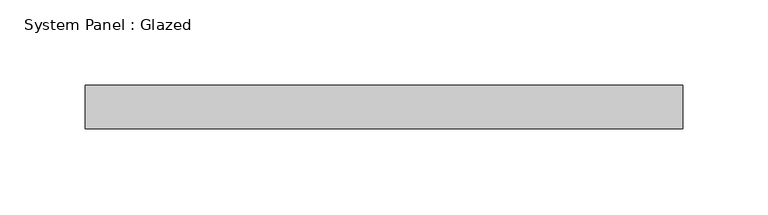
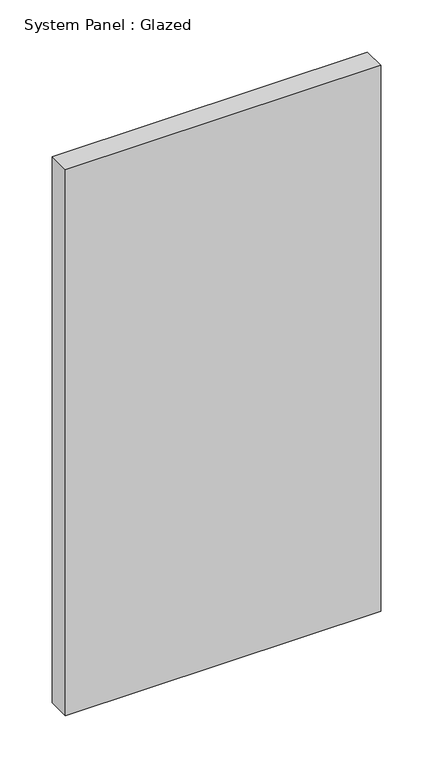
"""IFC4 building model written with IfcOpenShell, lengths in millimetres: plate geometry, System Panel : Glazed."""

from ifc_helpers import new_model, si_unit, origin, origin_with_axes, place, context, project, spatial, polyline, outline, extrude, source, transform, mapped, element, save


def system_panel_glazed_c3a15102(model_context):
    return source(origin(), model_context, "Body", "SweptSolid", [
        extrude(outline(polyline([(174.625, 19.05), (-174.625, 19.05), (-174.625, 44.45), (174.625, 44.45), (174.625, 19.05)])), origin_with_axes(), (0.0, 0.0, 1.0), 639.5466705),
    ])


if __name__ == "__main__":
    model = new_model("IFC4")
    model_context = context("Model", 3, world=origin())
    ifc_project = project(units=[si_unit("LENGTHUNIT", "METRE", prefix="MILLI")], contexts=[model_context])
    site = spatial("IfcSite", under=ifc_project)
    building = spatial("IfcBuilding", under=site)
    placement = place(None, origin())
    system_panel_glazed_shape = system_panel_glazed_c3a15102(model_context)
    element("IfcPlate", 1, ObjectType="System Panel : Glazed", at=placement, inside=building, context=model_context, shape_type="MappedRepresentation", body=[
        mapped(system_panel_glazed_shape, transform((0.0, 0.0, 0.0), x_axis=(1.0, 0.0, 0.0), y_axis=(0.0, 1.0, 0.0), z_axis=(0.0, 0.0, 1.0))),
    ])
    save(model, "model.ifc")

# Revit data of these elements
# Type "System Panel : Glazed"
#   Construction Type Id = "GSP4R"
#   Analytic Construction = "1/8 in Pilkington single glazing"
#   Visual Light Transmittance = 0.9
#   Solar Heat Gain Coefficient = 0.86
#   Heat Transfer Coefficient (U) = 1.18115 BTU/(h·ft²·°F)
#   Define Thermal Properties by = 1
# Element 1 (IfcPlate, "System Panel : Glazed")
#   Materials on its faces: "Glass"
# Materials
#   "Glass": class "Glass", colour RGB 0 128 192, transparency 0.75, Description = "Soda Lime Glass", Cost = 0
